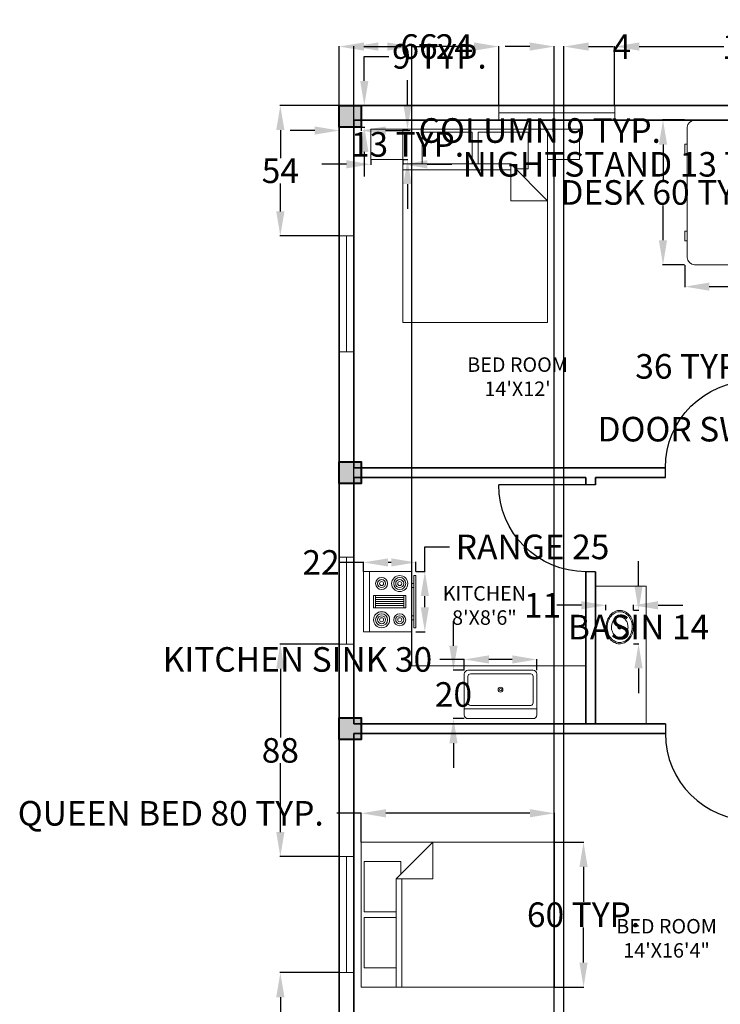
# Model space of a CAD drawing. Units: inches. Extents: x -107 to 647, y -210 to 500.
# Tile 2 of 7: x -107 to 183, y 92 to 500. Entities that reach past the tile are written whole.
import ezdxf

# ---------------------------------------------------------------- set-up
doc = ezdxf.new("R2010")
doc.units = ezdxf.units.IN
doc.header["$MEASUREMENT"] = 0
for name, color, linetype, lineweight in [('A-ANNO-DIMS', 2, 'Continuous', 18), ('A-AREA-IDEN', 7, 'Continuous', 18), ('A-COLS', 7, 'Continuous', 40), ('A-DOOR', 3, 'Continuous', 25), ('A-EQPM', 8, 'Continuous', 18), ('A-FLOR-CASE', 9, 'Continuous', 20), ('A-FLOR-FIXT', 9, 'Continuous', 18), ('A-FURN', 8, 'Continuous', 18), ('A-GLAZ', 4, 'Continuous', 18), ('A-WALL', 7, 'Continuous', 35)]:
    doc.layers.add(name, color=color, linetype=linetype, lineweight=lineweight)
doc.styles.get("Standard").update_dxf_attribs({"font": 'arial.ttf'})
doc.dimstyles.get("Standard").update_dxf_attribs({"dimtxt": 10.18, "dimasz": 10.18, "dimexe": 0.18, "dimexo": 0.0625, "dimgap": 0.09, "dimtad": 0, "dimtih": 1, "dimtoh": 1, "dimdec": 0, "dimzin": 0, "dimdsep": 46, "dimlunit": 3, "dimtxsty": 'Standard', "dimcen": 0.09, "dimadec": 0, "dimazin": 0, "dimtfac": 1, "dimtdec": 0, "dimtofl": 0, "dimtmove": 0, "dimatfit": 3, "dimfxl": 1, "dimtolj": 1, "dimtzin": 0, "dimarcsym": 0})

# ---------------------------------------------------------------- blocks, each defined once
blk = doc.blocks.new('Sink - Oval top')
for p, q in [((-1, 0), (1, 0)), ((0, 1), (0, -1))]:
    blk.add_line(p, q)
for points in [[(-12.23, 0.39, 0.117634), (-11.46, -3.36, 0.104469), (-8.88, -6.8, 0.090016), (-5.08, -9.07, 0.08192), (-0.32, -10.02, 0.08192), (4.49, -9.38, 0.090016), (8.42, -7.36, 0.104469), (11.22, -4.09, 0.117634), (12.23, -0.39, 0.117634), (11.46, 3.36, 0.104469), (8.88, 6.8, 0.090016), (5.08, 9.07, 0.08192), (0.32, 10.02, 0.08192), (-4.49, 9.38, 0.090016), (-8.42, 7.36, 0.104469), (-11.22, 4.09, 0.117634)], [(-11.29, 0.16, 0.118622), (-10.52, -3.25, 0.104678), (-8.07, -6.36, 0.089562), (-4.54, -8.37, 0.081185), (-0.13, -9.15, 0.081185), (4.3, -8.49, 0.089562), (7.89, -6.58, 0.104678), (10.42, -3.55, 0.118622), (11.29, -0.16, 0.118622), (10.52, 3.25, 0.104678), (8.07, 6.36, 0.089562), (4.54, 8.37, 0.081185), (0.13, 9.15, 0.081185), (-4.3, 8.49, 0.089562), (-7.89, 6.58, 0.104678), (-10.42, 3.55, 0.118622)], [(-7.42, 0.08, 0.118283), (-6.91, -2.17, 0.104607), (-5.29, -4.21, 0.089718), (-2.97, -5.53, 0.081436), (-0.07, -6.04, 0.081436), (2.84, -5.59, 0.089718), (5.2, -4.33, 0.104607), (6.86, -2.32, 0.118283), (7.42, -0.08, 0.118283), (6.91, 2.17, 0.104607), (5.29, 4.21, 0.089718), (2.97, 5.53, 0.081436), (0.07, 6.04, 0.081436), (-2.84, 5.59, 0.089718), (-5.2, 4.33, 0.104607), (-6.86, 2.32, 0.118283)]]:
    blk.add_lwpolyline(points, format="xyb", close=True)
for radius in [1.5, 1]:
    blk.add_circle((0, 0), radius)
blk = doc.blocks.new('Sink-single - 30 in top')
blk.add_line((-15, -3.999996), (15, -3.999996))
for points in [[(-13.5, 0), (13.5, 0)], [(-15, -18.499996), (-15, -1.5)], [(15, -1.5), (15, -18.499996)], [(-13.5, -17.499996), (-13.5, -6.499996)], [(-12.5, -5.499996), (12.5, -5.499996)], [(13.5, -6.499996), (13.5, -17.499996)], [(13.5, -19.999996), (-13.5, -19.999996)], [(12.5, -18.499996), (-12.5, -18.499996)]]:
    blk.add_lwpolyline(points)
for radius in [1, 0.5]:
    blk.add_circle((0, -11.999996), radius)
for centre, radius, start, end in [((-13.5, -1.5), 1.5, 90, 180), ((13.5, -1.5), 1.5, 0, 90), ((-12.5, -6.499996), 1, 90, 180), ((12.5, -6.499996), 1, 0, 90), ((-13.5, -18.499996), 1.5, 180, 270), ((-12.5, -17.499996), 1, 180, 270), ((12.5, -17.499996), 1, 270, 0), ((13.5, -18.499996), 1.5, 270, 0)]:
    blk.add_arc(centre, radius, start, end)
blk = doc.blocks.new('Range-Oven - 30 in top')
for p, q in [((0, -3), (30, -3)), ((12, -6), (18, -6)), ((13, -20), (13, -6)), ((14, -6), (14, -20)), ((15, -20), (15, -6)), ((16, -6), (16, -20)), ((17, -20), (17, -6)), ((6, -24), (6, -25)), ((8, -25), (8, -24)), ((18, -20), (12, -20)), ((22, -25), (22, -24)), ((24, -24), (24, -25))]:
    blk.add_line(p, q)
for points in [[(0, -24), (0, 0), (30, 0), (30, -24)], [(12, -21), (12, -5), (18, -5), (18, -21)], [(2, -26), (2, -25), (28, -25), (28, -26)]]:
    blk.add_lwpolyline(points, close=True)
for centre, radius in [((6, -9), 4), ((6, -9), 3), ((6, -9), 2), ((6, -9), 1), ((24, -9), 3), ((24, -9), 2), ((24, -9), 1), ((24, -18), 4), ((6, -18), 3), ((6, -18), 2), ((6, -18), 1), ((24, -18), 3), ((24, -18), 2), ((24, -18), 1)]:
    blk.add_circle(centre, radius)
blk = doc.blocks.new('Bed - Queen')
for p, q in [((0, -80.00003), (0, 0)), ((0, 0), (59.99999, 0)), ((59.99999, 0), (59.99999, -80.00003)), ((7.99999, -1.2), (28.79998, -1.2)), ((7.99999, -14.4), (7.99999, -1.2)), ((28.79998, -1.2), (28.79998, -14.4)), ((31.19999, -1.2), (51.99999, -1.2)), ((31.19999, -14.4), (31.19999, -1.2)), ((51.99999, -1.2), (51.99999, -16.4)), ((0, -14.4), (44.8, -14.4)), ((59.99999, -29.6), (44.8, -14.4)), ((44.8, -14.4), (44.8, -29.6)), ((44.8, -16.8), (0, -16.8)), ((51.99999, -16.4), (46.79936, -16.4)), ((44.8, -29.6), (59.99999, -29.6)), ((59.99999, -80.00003), (0, -80.00003))]:
    blk.add_line(p, q)
blk = doc.blocks.new('Desk - 30 x 60 in.')
for p, q in [((-26.999995, 0), (26.999995, 0)), ((-29.999995, -27), (-29.999995, -3)), ((29.999995, -3), (29.999995, -27)), ((26.999995, -30), (-26.999995, -30)), ((-20.000005, -30), (-20.000005, -31)), ((-20.000005, -31), (-16.000005, -31)), ((-16.000005, -31), (-16.000005, -30)), ((15.999995, -31), (15.999995, -30)), ((19.999995, -31), (15.999995, -31)), ((19.999995, -30), (19.999995, -31))]:
    blk.add_line(p, q)
for centre, start, end in [((-26.499995, -3.5), 98.1301, 171.8699), ((26.499995, -3.5), 8.130102, 81.8699), ((-26.499995, -26.5), 188.1301, 261.8699), ((26.499995, -26.5), 278.1301, 351.8699)]:
    blk.add_arc(centre, 3.535534, start, end)
blk = doc.blocks.new('DOOR-SWING-36IN')
for p, q in [((-36, 4), (-36, 0)), ((0, 4), (0, 0)), ((0, 0), (0, -36))]:
    blk.add_line(p, q)
blk.add_arc((0, 0), 36, 180, 270)
blk = doc.blocks.new('WINDOW-48IN')
for p, q in [((0, 6), (0, 0)), ((48, 6), (48, 0)), ((0, 3), (48, 3))]:
    blk.add_line(p, q)
blk = doc.blocks.new('WINDOW-36IN')
for p, q in [((0, 6), (0, 0)), ((36, 6), (36, 0)), ((0, 3), (36, 3))]:
    blk.add_line(p, q)
blk = doc.blocks.new('NIGHTSTAND-13IN')
blk.add_lwpolyline([(13.14, 12.56), (0, 12.56), (0, 0), (13.14, 0)], close=True)
blk = doc.blocks.new('COLUMN-9X9IN')
blk.add_lwpolyline([(0, 9), (9, 9), (9, 0), (0, 0)], close=True)
blk.add_solid([(0, 9), (0, 0), (9, 9), (9, 0)])
blk = doc.blocks.new('*D24')
at = {"layer": 'A-ANNO-DIMS', "color": 0, "lineweight": -2, "transparency": 16777216}
for p, q in [((14.9, 453.98), (4.72, 453.98)), ((25.08, 455.26), (25.08, 453.8)), ((34.08, 455.26), (34.08, 453.8)), ((44.26, 453.98), (54.44, 453.98))]:
    blk.add_line(p, q, dxfattribs=at)
at = {"layer": 'A-ANNO-DIMS', "color": 0, "transparency": 16777216}
for points in [[(14.9, 455.67), (14.9, 452.28), (25.08, 453.98)], [(44.26, 455.67), (44.26, 452.28), (34.08, 453.98)]]:
    blk.add_solid(points, dxfattribs=at)
at = {"layer": 'Defpoints', "color": 0, "transparency": 16777216}
for p in [(25.08, 455.33), (34.08, 455.33), (34.08, 453.98)]:
    blk.add_point(p, dxfattribs=at)
at = {"layer": 'A-ANNO-DIMS', "color": 0, "transparency": 16777216, "insert": (108.08, 453.98), "char_height": 10.18, "attachment_point": 5}
blk.add_mtext('\\A1;COLUMN 9 TYP.', dxfattribs=at)
blk = doc.blocks.new('*D25')
at = {"layer": 'A-ANNO-DIMS', "color": 0, "lineweight": -2, "transparency": 16777216}
for p, q in [((35.43, 474.51), (35.43, 484.69)), ((35.43, 484.69), (45.61, 484.69)), ((34.14, 464.33), (35.61, 464.33)), ((34.14, 455.33), (35.61, 455.33)), ((35.43, 445.15), (35.43, 434.97))]:
    blk.add_line(p, q, dxfattribs=at)
at = {"layer": 'A-ANNO-DIMS', "color": 0, "transparency": 16777216}
for points in [[(33.74, 474.51), (37.13, 474.51), (35.43, 464.33)], [(33.74, 445.15), (37.13, 445.15), (35.43, 455.33)]]:
    blk.add_solid(points, dxfattribs=at)
at = {"layer": 'Defpoints', "color": 0, "transparency": 16777216}
for p in [(34.08, 464.33), (35.43, 464.33), (34.08, 455.33)]:
    blk.add_point(p, dxfattribs=at)
at = {"layer": 'A-ANNO-DIMS', "color": 0, "transparency": 16777216, "insert": (66.52, 484.69), "char_height": 10.18, "attachment_point": 5}
blk.add_mtext('\\A1;9 TYP.', dxfattribs=at)
blk = doc.blocks.new('*D30')
at = {"layer": 'A-ANNO-DIMS', "color": 0, "lineweight": -2, "transparency": 16777216}
for p, q in [((206.02, 350.33), (199.9, 350.33)), ((200.08, 340.15), (200.08, 335.68)), ((200.08, 320.51), (200.08, 324.97)), ((206.02, 310.33), (199.9, 310.33))]:
    blk.add_line(p, q, dxfattribs=at)
at = {"layer": 'A-ANNO-DIMS', "color": 0, "transparency": 16777216}
for points in [[(198.39, 340.15), (201.78, 340.15), (200.08, 350.33)], [(198.39, 320.51), (201.78, 320.51), (200.08, 310.33)]]:
    blk.add_solid(points, dxfattribs=at)
at = {"layer": 'Defpoints', "color": 0, "transparency": 16777216}
for p in [(206.08, 350.33), (200.08, 310.33), (206.08, 310.33)]:
    blk.add_point(p, dxfattribs=at)
at = {"layer": 'A-ANNO-DIMS', "color": 0, "transparency": 16777216, "insert": (200.08, 330.33), "char_height": 10.18, "attachment_point": 5}
blk.add_mtext('\\A1;DOOR SWING 40 TYP.', dxfattribs=at)
blk = doc.blocks.new('*D31')
at = {"layer": 'A-ANNO-DIMS', "color": 0, "lineweight": -2, "transparency": 16777216}
for p, q in [((206.08, 356.33), (195.9, 356.33)), ((206.08, 350.39), (206.08, 356.51)), ((231.9, 356.33), (216.26, 356.33)), ((242.08, 350.39), (242.08, 356.51))]:
    blk.add_line(p, q, dxfattribs=at)
at = {"layer": 'A-ANNO-DIMS', "color": 0, "transparency": 16777216}
for points in [[(216.26, 358.02), (216.26, 354.63), (206.08, 356.33)], [(231.9, 358.02), (231.9, 354.63), (242.08, 356.33)]]:
    blk.add_solid(points, dxfattribs=at)
at = {"layer": 'Defpoints', "color": 0, "transparency": 16777216}
for p in [(206.08, 356.33), (206.08, 350.33), (242.08, 350.33)]:
    blk.add_point(p, dxfattribs=at)
at = {"layer": 'A-ANNO-DIMS', "color": 0, "transparency": 16777216, "insert": (171.04, 356.33), "char_height": 10.18, "attachment_point": 5}
blk.add_mtext('\\A1;36 TYP.', dxfattribs=at)
blk = doc.blocks.new('*D34')
at = {"layer": 'A-ANNO-DIMS', "color": 0, "lineweight": -2, "transparency": 16777216}
for p, q in [((148.96, 265.5), (148.96, 275.68)), ((146.94, 255.32), (149.14, 255.32)), ((146.94, 241.43), (149.14, 241.43)), ((148.96, 231.25), (148.96, 221.07))]:
    blk.add_line(p, q, dxfattribs=at)
at = {"layer": 'A-ANNO-DIMS', "color": 0, "transparency": 16777216}
for points in [[(147.27, 265.5), (150.66, 265.5), (148.96, 255.32)], [(147.27, 231.25), (150.66, 231.25), (148.96, 241.43)]]:
    blk.add_solid(points, dxfattribs=at)
at = {"layer": 'Defpoints', "color": 0, "transparency": 16777216}
for p in [(146.88, 255.32), (148.96, 255.32), (146.88, 241.43)]:
    blk.add_point(p, dxfattribs=at)
at = {"layer": 'A-ANNO-DIMS', "color": 0, "transparency": 16777216, "insert": (148.96, 248.38), "char_height": 10.18, "attachment_point": 5}
blk.add_mtext('\\A1;BASIN 14', dxfattribs=at)
blk = doc.blocks.new('*D35')
at = {"layer": 'A-ANNO-DIMS', "color": 0, "lineweight": -2, "transparency": 16777216}
for p, q in [((125.31, 257.41), (115.13, 257.41)), ((135.49, 255.38), (135.49, 257.59)), ((146.88, 255.38), (146.88, 257.59)), ((157.06, 257.41), (167.24, 257.41))]:
    blk.add_line(p, q, dxfattribs=at)
at = {"layer": 'A-ANNO-DIMS', "color": 0, "transparency": 16777216}
for points in [[(125.31, 259.1), (125.31, 255.71), (135.49, 257.41)], [(157.06, 259.1), (157.06, 255.71), (146.88, 257.41)]]:
    blk.add_solid(points, dxfattribs=at)
at = {"layer": 'Defpoints', "color": 0, "transparency": 16777216}
for p in [(135.49, 257.41), (135.49, 255.32), (146.88, 255.32)]:
    blk.add_point(p, dxfattribs=at)
at = {"layer": 'A-ANNO-DIMS', "color": 0, "transparency": 16777216, "insert": (109.21, 257.41), "char_height": 10.18, "attachment_point": 5}
blk.add_mtext('\\A1;11', dxfattribs=at)
blk = doc.blocks.new('*D40')
at = {"layer": 'A-ANNO-DIMS', "color": 0, "lineweight": -2, "transparency": 16777216}
for p, q in [((34.19, 171.29), (24.01, 171.29)), ((34.19, 159.36), (34.19, 171.47)), ((104.01, 171.29), (44.37, 171.29)), ((114.19, 159.36), (114.19, 171.47))]:
    blk.add_line(p, q, dxfattribs=at)
at = {"layer": 'A-ANNO-DIMS', "color": 0, "transparency": 16777216}
for points in [[(44.37, 172.99), (44.37, 169.6), (34.19, 171.29)], [(104.01, 172.99), (104.01, 169.6), (114.19, 171.29)]]:
    blk.add_solid(points, dxfattribs=at)
at = {"layer": 'Defpoints', "color": 0, "transparency": 16777216}
for p in [(34.19, 171.29), (34.19, 159.29), (114.19, 159.29)]:
    blk.add_point(p, dxfattribs=at)
at = {"layer": 'A-ANNO-DIMS', "color": 0, "transparency": 16777216, "insert": (-44.7, 171.29), "char_height": 10.18, "attachment_point": 5}
blk.add_mtext('\\A1;QUEEN BED 80 TYP.', dxfattribs=at)
blk = doc.blocks.new('*D41')
at = {"layer": 'A-ANNO-DIMS', "color": 0, "lineweight": -2, "transparency": 16777216}
for p, q in [((114.25, 159.29), (126.37, 159.29)), ((126.19, 149.11), (126.19, 134.58)), ((126.19, 109.47), (126.19, 124.01)), ((114.25, 99.29), (126.37, 99.29))]:
    blk.add_line(p, q, dxfattribs=at)
at = {"layer": 'A-ANNO-DIMS', "color": 0, "transparency": 16777216}
for points in [[(124.5, 149.11), (127.89, 149.11), (126.19, 159.29)], [(124.5, 109.47), (127.89, 109.47), (126.19, 99.29)]]:
    blk.add_solid(points, dxfattribs=at)
at = {"layer": 'Defpoints', "color": 0, "transparency": 16777216}
for p in [(114.19, 159.29), (126.19, 159.29), (114.19, 99.29)]:
    blk.add_point(p, dxfattribs=at)
at = {"layer": 'A-ANNO-DIMS', "color": 0, "transparency": 16777216, "insert": (126.19, 129.29), "char_height": 10.18, "attachment_point": 5}
blk.add_mtext('\\A1;60 TYP.', dxfattribs=at)
blk = doc.blocks.new('*D44')
at = {"layer": 'A-ANNO-DIMS', "color": 0, "lineweight": -2, "transparency": 16777216}
for p, q in [((168.03, 458.34), (158.91, 458.34)), ((159.09, 448.16), (159.09, 433.69)), ((159.09, 408.52), (159.09, 422.98)), ((168.03, 398.34), (158.91, 398.34))]:
    blk.add_line(p, q, dxfattribs=at)
at = {"layer": 'A-ANNO-DIMS', "color": 0, "transparency": 16777216}
for points in [[(157.39, 448.16), (160.78, 448.16), (159.09, 458.34)], [(157.39, 408.52), (160.78, 408.52), (159.09, 398.34)]]:
    blk.add_solid(points, dxfattribs=at)
at = {"layer": 'Defpoints', "color": 0, "transparency": 16777216}
for p in [(168.09, 458.34), (159.09, 398.34), (168.09, 398.34)]:
    blk.add_point(p, dxfattribs=at)
at = {"layer": 'A-ANNO-DIMS', "color": 0, "transparency": 16777216, "insert": (159.09, 428.34), "char_height": 10.18, "attachment_point": 5}
blk.add_mtext('\\A1;DESK 60 TYP.', dxfattribs=at)
blk = doc.blocks.new('*D45')
at = {"layer": 'A-ANNO-DIMS', "color": 0, "lineweight": -2, "transparency": 16777216}
for p, q in [((168.09, 398.27), (168.09, 389.16)), ((199.09, 398.27), (199.09, 389.16)), ((178.27, 389.34), (188.91, 389.34)), ((199.09, 389.34), (209.27, 389.34))]:
    blk.add_line(p, q, dxfattribs=at)
at = {"layer": 'A-ANNO-DIMS', "color": 0, "transparency": 16777216}
for points in [[(178.27, 391.03), (178.27, 387.64), (168.09, 389.34)], [(188.91, 391.03), (188.91, 387.64), (199.09, 389.34)]]:
    blk.add_solid(points, dxfattribs=at)
at = {"layer": 'Defpoints', "color": 0, "transparency": 16777216}
for p in [(168.09, 398.34), (199.09, 398.34), (199.09, 389.34)]:
    blk.add_point(p, dxfattribs=at)
at = {"layer": 'A-ANNO-DIMS', "color": 0, "transparency": 16777216, "insert": (234.13, 389.34), "char_height": 10.18, "attachment_point": 5}
blk.add_mtext('\\A1;31 TYP.', dxfattribs=at)
blk = doc.blocks.new('*D50')
at = {"layer": 'A-ANNO-DIMS', "color": 0, "lineweight": -2, "transparency": 16777216}
for p, q in [((38.19, 441.9), (38.19, 439.81)), ((51.33, 441.9), (51.33, 439.81)), ((28.01, 439.99), (17.83, 439.99)), ((61.51, 439.99), (71.69, 439.99))]:
    blk.add_line(p, q, dxfattribs=at)
at = {"layer": 'A-ANNO-DIMS', "color": 0, "transparency": 16777216}
for points in [[(28.01, 441.69), (28.01, 438.29), (38.19, 439.99)], [(61.51, 441.69), (61.51, 438.29), (51.33, 439.99)]]:
    blk.add_solid(points, dxfattribs=at)
at = {"layer": 'Defpoints', "color": 0, "transparency": 16777216}
for p in [(38.19, 441.96), (51.33, 441.96), (51.33, 439.99)]:
    blk.add_point(p, dxfattribs=at)
at = {"layer": 'A-ANNO-DIMS', "color": 0, "transparency": 16777216, "insert": (144.5, 439.99), "char_height": 10.18, "attachment_point": 5}
blk.add_mtext('\\A1;NIGHTSTAND 13 TYP.', dxfattribs=at)
blk = doc.blocks.new('*D51')
at = {"layer": 'A-ANNO-DIMS', "color": 0, "lineweight": -2, "transparency": 16777216}
for p, q in [((53.3, 464.7), (53.3, 474.88)), ((51.39, 454.52), (53.48, 454.52)), ((51.39, 441.96), (53.48, 441.96)), ((53.3, 431.78), (53.3, 421.6))]:
    blk.add_line(p, q, dxfattribs=at)
at = {"layer": 'A-ANNO-DIMS', "color": 0, "transparency": 16777216}
for points in [[(51.6, 464.7), (55, 464.7), (53.3, 454.52)], [(51.6, 431.78), (55, 431.78), (53.3, 441.96)]]:
    blk.add_solid(points, dxfattribs=at)
at = {"layer": 'Defpoints', "color": 0, "transparency": 16777216}
for p in [(51.33, 454.52), (53.3, 454.52), (51.33, 441.96)]:
    blk.add_point(p, dxfattribs=at)
at = {"layer": 'A-ANNO-DIMS', "color": 0, "transparency": 16777216, "insert": (53.3, 448.24), "char_height": 10.18, "attachment_point": 5}
blk.add_mtext('\\A1;13 TYP.', dxfattribs=at)
blk = doc.blocks.new('*D62')
at = {"layer": 'A-ANNO-DIMS', "color": 0, "lineweight": -2, "transparency": 16777216}
for p, q in [((76.84, 234.98), (66.66, 234.98)), ((76.84, 230.54), (76.84, 235.16)), ((96.66, 234.98), (87.02, 234.98)), ((106.84, 230.54), (106.84, 235.16))]:
    blk.add_line(p, q, dxfattribs=at)
at = {"layer": 'A-ANNO-DIMS', "color": 0, "transparency": 16777216}
for points in [[(87.02, 236.68), (87.02, 233.28), (76.84, 234.98)], [(96.66, 236.68), (96.66, 233.28), (106.84, 234.98)]]:
    blk.add_solid(points, dxfattribs=at)
at = {"layer": 'Defpoints', "color": 0, "transparency": 16777216}
for p in [(76.84, 234.98), (76.84, 230.48), (106.84, 230.48)]:
    blk.add_point(p, dxfattribs=at)
at = {"layer": 'A-ANNO-DIMS', "color": 0, "transparency": 16777216, "insert": (7.76, 234.98), "char_height": 10.18, "attachment_point": 5}
blk.add_mtext('\\A1;KITCHEN SINK 30', dxfattribs=at)
blk = doc.blocks.new('*D63')
at = {"layer": 'A-ANNO-DIMS', "color": 0, "lineweight": -2, "transparency": 16777216}
for p, q in [((72.34, 240.66), (72.34, 250.84)), ((76.77, 230.48), (72.16, 230.48)), ((76.77, 210.48), (72.16, 210.48)), ((72.34, 200.3), (72.34, 190.12))]:
    blk.add_line(p, q, dxfattribs=at)
at = {"layer": 'A-ANNO-DIMS', "color": 0, "transparency": 16777216}
for points in [[(70.64, 240.66), (74.03, 240.66), (72.34, 230.48)], [(70.64, 200.3), (74.03, 200.3), (72.34, 210.48)]]:
    blk.add_solid(points, dxfattribs=at)
at = {"layer": 'Defpoints', "color": 0, "transparency": 16777216}
for p in [(76.84, 230.48), (72.34, 210.48), (76.84, 210.48)]:
    blk.add_point(p, dxfattribs=at)
at = {"layer": 'A-ANNO-DIMS', "color": 0, "transparency": 16777216, "insert": (72.34, 220.48), "char_height": 10.18, "attachment_point": 5}
blk.add_mtext('\\A1;20', dxfattribs=at)
blk = doc.blocks.new('*D64')
at = {"layer": 'A-ANNO-DIMS', "color": 0, "lineweight": -2, "transparency": 16777216}
for p, q in [((60.49, 271.4), (60.49, 281.58)), ((60.49, 281.58), (70.67, 281.58)), ((56.81, 271.4), (60.67, 271.4)), ((60.49, 256.61), (60.49, 261.22)), ((56.81, 246.43), (60.67, 246.43))]:
    blk.add_line(p, q, dxfattribs=at)
at = {"layer": 'A-ANNO-DIMS', "color": 0, "transparency": 16777216}
for points in [[(58.8, 261.22), (62.19, 261.22), (60.49, 271.4)], [(58.8, 256.61), (62.19, 256.61), (60.49, 246.43)]]:
    blk.add_solid(points, dxfattribs=at)
at = {"layer": 'Defpoints', "color": 0, "transparency": 16777216}
for p in [(56.75, 271.4), (60.49, 271.4), (56.75, 246.43)]:
    blk.add_point(p, dxfattribs=at)
at = {"layer": 'A-ANNO-DIMS', "color": 0, "transparency": 16777216, "insert": (105.09, 281.58), "char_height": 10.18, "attachment_point": 5}
blk.add_mtext('\\A1;RANGE 25', dxfattribs=at)
blk = doc.blocks.new('*D65')
at = {"layer": 'A-ANNO-DIMS', "color": 0, "lineweight": -2, "transparency": 16777216}
for p, q in [((35.11, 275.15), (24.93, 275.15)), ((35.11, 271.46), (35.11, 275.33)), ((46.57, 275.15), (45.29, 275.15)), ((56.75, 271.46), (56.75, 275.33))]:
    blk.add_line(p, q, dxfattribs=at)
at = {"layer": 'A-ANNO-DIMS', "color": 0, "transparency": 16777216}
for points in [[(45.29, 276.84), (45.29, 273.45), (35.11, 275.15)], [(46.57, 276.84), (46.57, 273.45), (56.75, 275.15)]]:
    blk.add_solid(points, dxfattribs=at)
at = {"layer": 'Defpoints', "color": 0, "transparency": 16777216}
for p in [(35.11, 275.15), (35.11, 271.4), (56.75, 271.4)]:
    blk.add_point(p, dxfattribs=at)
at = {"layer": 'A-ANNO-DIMS', "color": 0, "transparency": 16777216, "insert": (17.51, 275.15), "char_height": 10.18, "attachment_point": 5}
blk.add_mtext('\\A1;22', dxfattribs=at)
blk = doc.blocks.new('*D75')
at = {"layer": 'A-ANNO-DIMS', "color": 0, "lineweight": -2, "transparency": 16777216}
for p, q in [((25.08, 464.39), (25.08, 488.92)), ((35.26, 488.74), (50.68, 488.74)), ((80.9, 488.74), (65.49, 488.74)), ((91.08, 464.39), (91.08, 488.92))]:
    blk.add_line(p, q, dxfattribs=at)
at = {"layer": 'A-ANNO-DIMS', "color": 0, "transparency": 16777216}
for points in [[(35.26, 490.44), (35.26, 487.04), (25.08, 488.74)], [(80.9, 490.44), (80.9, 487.04), (91.08, 488.74)]]:
    blk.add_solid(points, dxfattribs=at)
at = {"layer": 'Defpoints', "color": 0, "transparency": 16777216}
for p in [(91.08, 488.74), (25.08, 464.33), (91.08, 464.33)]:
    blk.add_point(p, dxfattribs=at)
at = {"layer": 'A-ANNO-DIMS', "color": 0, "transparency": 16777216, "insert": (58.08, 488.74), "char_height": 10.18, "attachment_point": 5}
blk.add_mtext('\\A1;66', dxfattribs=at)
blk = doc.blocks.new('*D76')
at = {"layer": 'A-ANNO-DIMS', "color": 0, "lineweight": -2, "transparency": 16777216}
for p, q in [((139.08, 464.39), (139.08, 488.92)), ((149.26, 488.74), (184.28, 488.74)), ((240.9, 488.74), (205.89, 488.74)), ((251.08, 464.39), (251.08, 488.92))]:
    blk.add_line(p, q, dxfattribs=at)
at = {"layer": 'A-ANNO-DIMS', "color": 0, "transparency": 16777216}
for points in [[(149.26, 490.44), (149.26, 487.04), (139.08, 488.74)], [(240.9, 490.44), (240.9, 487.04), (251.08, 488.74)]]:
    blk.add_solid(points, dxfattribs=at)
at = {"layer": 'Defpoints', "color": 0, "transparency": 16777216}
for p in [(251.08, 488.74), (139.08, 464.33), (251.08, 464.33)]:
    blk.add_point(p, dxfattribs=at)
at = {"layer": 'A-ANNO-DIMS', "color": 0, "transparency": 16777216, "insert": (195.08, 488.74), "char_height": 10.18, "attachment_point": 5}
blk.add_mtext('\\A1;112', dxfattribs=at)
blk = doc.blocks.new('*D77')
at = {"layer": 'A-ANNO-DIMS', "color": 0, "lineweight": -2, "transparency": 16777216}
for p, q in [((25.02, 464.33), (0.49, 464.33)), ((0.67, 454.15), (0.67, 442.59)), ((0.67, 420.51), (0.67, 432.06)), ((25.02, 410.33), (0.49, 410.33))]:
    blk.add_line(p, q, dxfattribs=at)
at = {"layer": 'A-ANNO-DIMS', "color": 0, "transparency": 16777216}
for points in [[(-1.03, 454.15), (2.36, 454.15), (0.67, 464.33)], [(-1.03, 420.51), (2.36, 420.51), (0.67, 410.33)]]:
    blk.add_solid(points, dxfattribs=at)
at = {"layer": 'Defpoints', "color": 0, "transparency": 16777216}
for p in [(25.08, 464.33), (0.67, 410.33), (25.08, 410.33)]:
    blk.add_point(p, dxfattribs=at)
at = {"layer": 'A-ANNO-DIMS', "color": 0, "transparency": 16777216, "insert": (0.67, 437.33), "char_height": 10.18, "attachment_point": 5}
blk.add_mtext('\\A1;54', dxfattribs=at)
blk = doc.blocks.new('*D78')
at = {"layer": 'A-ANNO-DIMS', "color": 0, "lineweight": -2, "transparency": 16777216}
for p, q in [((25.02, 241.33), (0.49, 241.33)), ((0.67, 231.15), (0.67, 202.61)), ((0.67, 163.51), (0.67, 192.04)), ((25.02, 153.33), (0.49, 153.33))]:
    blk.add_line(p, q, dxfattribs=at)
at = {"layer": 'A-ANNO-DIMS', "color": 0, "transparency": 16777216}
for points in [[(-1.03, 231.15), (2.36, 231.15), (0.67, 241.33)], [(-1.03, 163.51), (2.36, 163.51), (0.67, 153.33)]]:
    blk.add_solid(points, dxfattribs=at)
at = {"layer": 'Defpoints', "color": 0, "transparency": 16777216}
for p in [(25.08, 241.33), (0.67, 153.33), (25.08, 153.33)]:
    blk.add_point(p, dxfattribs=at)
at = {"layer": 'A-ANNO-DIMS', "color": 0, "transparency": 16777216, "insert": (0.67, 197.33), "char_height": 10.18, "attachment_point": 5}
blk.add_mtext('\\A1;88', dxfattribs=at)
blk = doc.blocks.new('*D79')
at = {"layer": 'A-ANNO-DIMS', "color": 0, "lineweight": -2, "transparency": 16777216}
for p, q in [((25.02, 105.33), (0.49, 105.33)), ((0.67, 95.15), (0.67, 59.12)), ((0.67, 12.51), (0.67, 48.53)), ((25.02, 2.33), (0.49, 2.33))]:
    blk.add_line(p, q, dxfattribs=at)
at = {"layer": 'A-ANNO-DIMS', "color": 0, "transparency": 16777216}
for points in [[(-1.03, 95.15), (2.36, 95.15), (0.67, 105.33)], [(-1.03, 12.51), (2.36, 12.51), (0.67, 2.33)]]:
    blk.add_solid(points, dxfattribs=at)
at = {"layer": 'Defpoints', "color": 0, "transparency": 16777216}
for p in [(0.67, 105.33), (25.08, 105.33), (25.08, 2.33)]:
    blk.add_point(p, dxfattribs=at)
at = {"layer": 'A-ANNO-DIMS', "color": 0, "transparency": 16777216, "insert": (0.67, 53.83), "char_height": 10.18, "attachment_point": 5}
blk.add_mtext('\\A1;103', dxfattribs=at)
blk = doc.blocks.new('*D82')
at = {"layer": 'A-ANNO-DIMS', "color": 0, "lineweight": -2, "transparency": 16777216}
for p, q in [((103.9, 488.74), (93.72, 488.74)), ((114.08, 50.39), (114.08, 488.92)), ((118.08, 54.39), (118.08, 488.92)), ((128.26, 488.74), (138.44, 488.74))]:
    blk.add_line(p, q, dxfattribs=at)
at = {"layer": 'A-ANNO-DIMS', "color": 0, "transparency": 16777216}
for points in [[(103.9, 490.44), (103.9, 487.04), (114.08, 488.74)], [(128.26, 490.44), (128.26, 487.04), (118.08, 488.74)]]:
    blk.add_solid(points, dxfattribs=at)
at = {"layer": 'Defpoints', "color": 0, "transparency": 16777216}
for p in [(118.08, 488.74), (118.08, 54.33), (114.08, 50.33)]:
    blk.add_point(p, dxfattribs=at)
at = {"layer": 'A-ANNO-DIMS', "color": 0, "transparency": 16777216, "insert": (142.05, 488.74), "char_height": 10.18, "attachment_point": 5}
blk.add_mtext('\\A1;4', dxfattribs=at)
blk = doc.blocks.new('*D83')
at = {"layer": 'A-ANNO-DIMS', "color": 0, "lineweight": -2, "transparency": 16777216}
for p, q in [((31.08, 208.39), (31.08, 488.92)), ((41.26, 488.74), (44.9, 488.74)), ((55.08, 232.39), (55.08, 488.92)), ((55.08, 488.74), (65.26, 488.74))]:
    blk.add_line(p, q, dxfattribs=at)
at = {"layer": 'A-ANNO-DIMS', "color": 0, "transparency": 16777216}
for points in [[(41.26, 490.44), (41.26, 487.04), (31.08, 488.74)], [(44.9, 490.44), (44.9, 487.04), (55.08, 488.74)]]:
    blk.add_solid(points, dxfattribs=at)
at = {"layer": 'Defpoints', "color": 0, "transparency": 16777216}
for p in [(55.08, 488.74), (55.08, 232.33), (31.08, 208.33)]:
    blk.add_point(p, dxfattribs=at)
at = {"layer": 'A-ANNO-DIMS', "color": 0, "transparency": 16777216, "insert": (72.71, 488.74), "char_height": 10.18, "attachment_point": 5}
blk.add_mtext('\\A1;24', dxfattribs=at)

msp = doc.modelspace()

# ---------------------------------------------------------------- linework, layer by layer
at = {"layer": 'A-FLOR-CASE'}
for p, q in [((55.082, 310.325), (55.082, 232.325)), ((152.082, 265.325), (131.082, 265.325)), ((152.082, 265.325), (152.082, 208.325)), ((127.082, 232.325), (55.082, 232.325))]:
    msp.add_line(p, q, dxfattribs=at)
at = {"layer": 'A-WALL'}
for p, q in [((31.082, 458.325), (31.082, 314.325)), ((199.082, 458.325), (31.082, 458.325)), ((160.082, 314.325), (31.082, 314.325)), ((127.082, 310.325), (31.082, 310.325)), ((31.082, 310.325), (31.082, 208.325)), ((127.082, 310.325), (127.082, 307.325)), ((131.082, 310.325), (131.082, 307.325)), ((160.082, 310.325), (131.082, 310.325)), ((127.082, 271.325), (127.082, 208.325)), ((131.082, 271.325), (131.082, 208.325)), ((160.082, 208.325), (31.082, 208.325)), ((31.082, 204.325), (31.082, 54.325)), ((160.082, 204.325), (31.082, 204.325))]:
    msp.add_line(p, q, dxfattribs=at)
msp.add_lwpolyline([(25.082, 2.325), (409.082, 2.325), (409.082, 464.325), (25.082, 464.325)], close=True, dxfattribs=at)

# ---------------------------------------------------------------- block references
at = {"layer": 'A-COLS'}
for p in [(25.082, 455.325), (25.082, 307.843), (25.082, 201.864)]:
    msp.add_blockref('COLUMN-9X9IN', p, dxfattribs=at)
at = {"layer": 'A-DOOR', "extrusion": (0, 0, -1), "zscale": -1}
for p, rotation in [((-196.082, 314.325), 180), ((-127.082, 307.325), 89.99999999999999)]:
    msp.add_blockref('DOOR-SWING-36IN', p, dxfattribs=dict(at, rotation=rotation))
at = {"layer": 'A-DOOR'}
msp.add_blockref('DOOR-SWING-36IN', (196.082, 204.325), dxfattribs=at)
at = {"layer": 'A-EQPM', "xscale": 0.8323519030541284, "yscale": 0.8323519030541284, "zscale": 0.8323519030541284, "rotation": 90}
msp.add_blockref('Range-Oven - 30 in top', (35.105, 246.429), dxfattribs=at)
at = {"layer": 'A-FLOR-FIXT', "xscale": 0.5657208398595476, "yscale": 0.5657208398595476, "zscale": 0.5657208398595476, "rotation": 90}
msp.add_blockref('Sink - Oval top', (141.184, 248.377), dxfattribs=at)
at = {"layer": 'A-FLOR-FIXT', "rotation": 180}
msp.add_blockref('Sink-single - 30 in top', (91.837, 210.482), dxfattribs=at)
at = {"layer": 'A-FURN'}
for name, p, rotation in [('Desk - 30 x 60 in.', (199.088, 428.336), 270), ('Bed - Queen', (34.192, 99.294), 90)]:
    msp.add_blockref(name, p, dxfattribs=dict(at, rotation=rotation))
for name, p in [('NIGHTSTAND-13IN', (38.19, 441.959)), ('Bed - Queen', (51.328, 454.519))]:
    msp.add_blockref(name, p, dxfattribs=at)
at = {"layer": 'A-FURN', "extrusion": (0, 0, -1), "zscale": -1}
msp.add_blockref('NIGHTSTAND-13IN', (-124.466, 441.959), dxfattribs=at)
at = {"layer": 'A-GLAZ'}
msp.add_blockref('WINDOW-48IN', (91.082, 458.325), dxfattribs=at)
for name, p, rotation in [('WINDOW-48IN', (31.082, 362.325), 89.99999999999972), ('WINDOW-36IN', (31.082, 241.325), 89.99999999999991), ('WINDOW-48IN', (31.082, 105.325), 89.99999999999972)]:
    msp.add_blockref(name, p, dxfattribs=dict(at, rotation=rotation))

# ---------------------------------------------------------------- texts
at = {"layer": 'A-AREA-IDEN', "char_height": 6, "attachment_point": 1}
for s, width, insert in [("\\pxqc;BED ROOM\\P14'X12'", 45.88849, (75.932, 360.058)), ('\\pxqc;KITCHEN\\P8\'X8\'6"', 36.24576, (67.032, 265.325)), ('\\pxqc;BED ROOM\\P14\'X16\'4"', 45.88849, (137.611, 127.515))]:
    msp.add_mtext_dynamic_manual_height_columns(s, width=width, gutter_width=1, heights=[0], dxfattribs=dict(at, insert=insert))

# ---------------------------------------------------------------- dimensions: what is measured, and where the dimension line sits
at = {"layer": 'A-ANNO-DIMS'}
for base, p1, p2, angle, text, picture, middle in [((35.432, 464.325), (34.082, 455.325), (34.082, 464.325), 90, '<> TYP.', '*D25', (66.523, 484.685)), ((53.299, 454.519), (51.328, 441.959), (51.328, 454.519), 90, '<> TYP.', '*D51', (53.299, 448.239)), ((159.088, 398.336), (168.088, 458.336), (168.088, 398.336), 270, 'DESK <> TYP.', '*D44', (159.088, 428.336)), ((206.082, 356.325), (242.082, 350.325), (206.082, 350.325), 180, '<> TYP.', '*D31', (171.039, 356.325)), ((200.082, 310.325), (206.082, 350.325), (206.082, 310.325), 270, 'DOOR SWING <> TYP.', '*D30', (200.082, 330.325)), ((60.492, 271.4), (56.746, 246.429), (56.746, 271.4), 90, 'RANGE <>', '*D64', (105.09, 281.58)), ((148.964, 255.322), (146.88, 241.433), (146.88, 255.322), 90, 'BASIN <>', '*D34', (148.964, 248.377)), ((76.837, 234.982), (106.837, 230.482), (76.837, 230.482), 180, 'KITCHEN SINK <>', '*D62', (7.761, 234.982)), ((34.192, 171.294), (114.192, 159.294), (34.192, 159.294), 180, 'QUEEN BED <> TYP.', '*D40', (-44.703, 171.294)), ((126.192, 159.294), (114.192, 99.294), (114.192, 159.294), 90, '<> TYP.', '*D41', (126.192, 129.294))]:
    dim = msp.add_linear_dim(base=base, p1=p1, p2=p2, angle=angle, text=text, dimstyle='Standard', override={"dimdec": 0, "dimlfac": 1, "dimrnd": 0, "dimzin": 0, "dimdsep": 46, "dimlunit": 2}, dxfattribs=at)
    dim.commit()
    dim.dimension.update_dxf_attribs({"geometry": picture, "text_midpoint": middle})
for base, p1, p2, picture, middle in [((91.082, 488.742), (25.082, 464.325), (91.082, 464.325), '*D75', (58.082, 488.742)), ((55.082, 488.742), (31.082, 208.325), (55.082, 232.325), '*D83', (72.709, 488.742)), ((118.082, 488.742), (114.082, 50.325), (118.082, 54.325), '*D82', (142.052, 488.742)), ((251.082, 488.742), (139.082, 464.325), (251.082, 464.325), '*D76', (195.082, 488.742))]:
    dim = msp.add_linear_dim(base=base, p1=p1, p2=p2, dimstyle='Standard', override={"dimdec": 0, "dimlfac": 1, "dimrnd": 0, "dimzin": 0, "dimdsep": 46, "dimlunit": 2}, dxfattribs=at)
    dim.commit()
    dim.dimension.update_dxf_attribs({"geometry": picture, "text_midpoint": middle})
for base, p1, p2, text, picture, middle in [((34.082, 453.975), (25.082, 455.325), (34.082, 455.325), 'COLUMN <> TYP.', '*D24', (108.084, 453.975)), ((51.328, 439.989), (38.19, 441.959), (51.328, 441.959), 'NIGHTSTAND <> TYP.', '*D50', (144.503, 439.989)), ((199.088, 389.336), (168.088, 398.336), (199.088, 398.336), '<> TYP.', '*D45', (234.131, 389.336))]:
    dim = msp.add_linear_dim(base=base, p1=p1, p2=p2, text=text, dimstyle='Standard', override={"dimdec": 0, "dimlfac": 1, "dimrnd": 0, "dimzin": 0, "dimdsep": 46, "dimlunit": 2}, dxfattribs=at)
    dim.commit()
    dim.dimension.update_dxf_attribs({"geometry": picture, "text_midpoint": middle})
for base, p1, p2, angle, picture, middle in [((0.665, 410.325), (25.082, 464.325), (25.082, 410.325), 90, '*D77', (0.665, 437.325)), ((35.105, 275.145), (56.746, 271.4), (35.105, 271.4), 180, '*D65', (17.509, 275.145)), ((135.489, 257.405), (146.88, 255.322), (135.489, 255.322), 180, '*D35', (109.209, 257.405)), ((72.337, 210.482), (76.837, 230.482), (76.837, 210.482), 270, '*D63', (72.337, 220.482)), ((0.665, 153.325), (25.082, 241.325), (25.082, 153.325), 90, '*D78', (0.665, 197.325)), ((0.665, 105.325), (25.082, 2.325), (25.082, 105.325), 90, '*D79', (0.665, 53.825))]:
    dim = msp.add_linear_dim(base=base, p1=p1, p2=p2, angle=angle, dimstyle='Standard', override={"dimdec": 0, "dimlfac": 1, "dimrnd": 0, "dimzin": 0, "dimdsep": 46, "dimlunit": 2}, dxfattribs=at)
    dim.commit()
    dim.dimension.update_dxf_attribs({"geometry": picture, "text_midpoint": middle})

doc.saveas('drawing.dxf')
